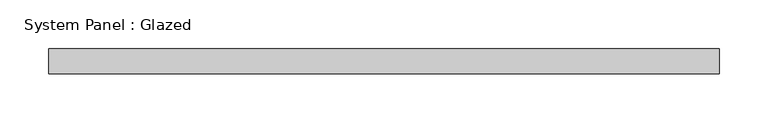
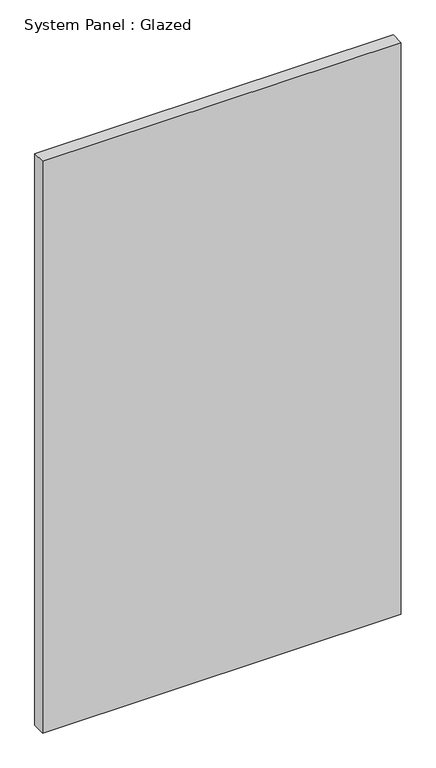
"""IFC4 building model written with IfcOpenShell, lengths in millimetres: plate geometry, System Panel : Glazed."""

from ifc_helpers import new_model, si_unit, origin, origin_with_axes, place, context, project, spatial, polyline, outline, extrude, source, transform, mapped, element, save


def system_panel_glazed_a1f4a93c(model_context):
    return source(origin(), model_context, "Body", "SweptSolid", [
        extrude(outline(polyline([(342.9, 19.05), (-342.9, 19.05), (-342.9, 44.45), (342.9, 44.45), (342.9, 19.05)])), origin_with_axes(), (0.0, 0.0, 1.0), 1155.7),
    ])


if __name__ == "__main__":
    model = new_model("IFC4")
    model_context = context("Model", 3, world=origin())
    ifc_project = project(units=[si_unit("LENGTHUNIT", "METRE", prefix="MILLI")], contexts=[model_context])
    site = spatial("IfcSite", under=ifc_project)
    building = spatial("IfcBuilding", under=site)
    placement = place(None, origin())
    system_panel_glazed_shape = system_panel_glazed_a1f4a93c(model_context)
    element("IfcPlate", 1, ObjectType="System Panel : Glazed", at=placement, inside=building, context=model_context, shape_type="MappedRepresentation", body=[
        mapped(system_panel_glazed_shape, transform((0.0, 0.0, 0.0), x_axis=(1.0, 0.0, 0.0), y_axis=(0.0, 1.0, 0.0), z_axis=(0.0, 0.0, 1.0))),
    ])
    save(model, "model.ifc")

# Revit data of these elements
# Type "System Panel : Glazed"
#   Construction Type Id = "GSP4R"
#   Analytic Construction = "1/8 in Pilkington single glazing"
#   Visual Light Transmittance = 0.9
#   Solar Heat Gain Coefficient = 0.86
#   Heat Transfer Coefficient (U) = 1.18115 BTU/(h·ft²·°F)
# Element 1 (IfcPlate, "System Panel : Glazed")
#   Materials on its faces: "Glass"
# Materials
#   "Glass": class "Glass", colour RGB 0 128 192, transparency 0.75, Description = "Soda Lime Glass", Cost = 0
